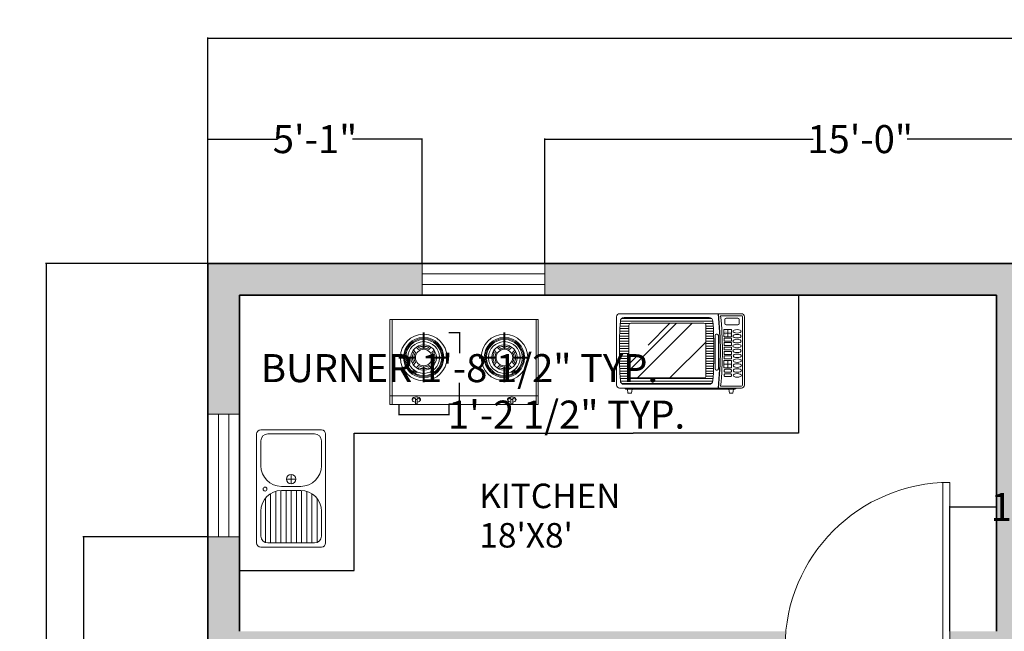
# Model space of a CAD drawing. Units: inches. Extents: x 638 to 1303, y 1 to 699.
# Tile 11 of 21: x 644 to 924, y 525 to 699. Entities that reach past the tile are written whole.
import ezdxf

# ---------------------------------------------------------------- set-up
doc = ezdxf.new("R2010")
doc.units = ezdxf.units.IN
doc.header["$MEASUREMENT"] = 0
for name, color, linetype, lineweight in [('A-ANNO-DIMS', 2, 'Continuous', 18), ('A-AREA-IDEN', 7, 'Continuous', 18), ('A-DOOR', 4, 'Continuous', 18), ('A-EQPM', 8, 'Continuous', 15), ('A-EQPM-PATT', 8, 'Continuous', 13), ('A-EQPM-TEXT', 8, 'Continuous', 13), ('A-FLOR-CASE', 8, 'Continuous', 25), ('A-FLOR-FIXT', 9, 'Continuous', 18), ('A-GLAZ', 4, 'Continuous', 18), ('A-WALL', 7, 'Continuous', 35)]:
    doc.layers.add(name, color=color, linetype=linetype, lineweight=lineweight)
doc.layers.add('A-WALL-PATT', color=143, linetype='Continuous', lineweight=13, true_color=0x7aafdf)
doc.styles.get("Standard").update_dxf_attribs({"font": 'arial.ttf'})
doc.dimstyles.get("Standard").update_dxf_attribs({"dimtxt": 8, "dimasz": 0.18, "dimexe": 0.18, "dimexo": 0.0625, "dimgap": 0.09, "dimtad": 0, "dimtih": 1, "dimtoh": 1, "dimdec": 4, "dimzin": 0, "dimdsep": 46, "dimlunit": 3, "dimtxsty": 'Standard', "dimcen": 0.09, "dimadec": 0, "dimazin": 0, "dimtfac": 1, "dimtdec": 4, "dimtofl": 0, "dimtmove": 0, "dimatfit": 3, "dimfxl": 1, "dimtolj": 1, "dimtzin": 0, "dimarcsym": 0})

# ---------------------------------------------------------------- blocks, each defined once
blk = doc.blocks.new('*D1')
at = {"layer": 'A-ANNO-DIMS', "color": 0, "lineweight": -2, "transparency": 16777216}
for p, q in [((697.18, 629.82), (650.92, 629.82)), ((651.1, 629.64), (651.1, 339.99)), ((651.1, 42), (651.1, 331.64)), ((697.18, 41.82), (650.92, 41.82))]:
    blk.add_line(p, q, dxfattribs=at)
at = {"layer": 'A-ANNO-DIMS', "color": 0, "transparency": 16777216}
for points in [[(651.07, 629.64), (651.13, 629.64), (651.1, 629.82)], [(651.07, 42), (651.13, 42), (651.1, 41.82)]]:
    blk.add_solid(points, dxfattribs=at)
at = {"layer": 'Defpoints', "color": 0, "transparency": 16777216}
for p in [(697.24, 629.82), (651.1, 41.82), (697.24, 41.82)]:
    blk.add_point(p, dxfattribs=at)
at = {"layer": 'A-ANNO-DIMS', "color": 0, "transparency": 16777216, "insert": (651.1, 335.82), "char_height": 8, "attachment_point": 5}
blk.add_mtext("\\A1;49'", dxfattribs=at)
blk = doc.blocks.new('*D2')
at = {"layer": 'A-ANNO-DIMS', "color": 0, "lineweight": -2, "transparency": 16777216}
for p, q in [((697.24, 629.88), (697.24, 694.35)), ((697.42, 694.17), (934.76, 694.17)), ((1228.06, 694.17), (990.71, 694.17)), ((1228.24, 629.88), (1228.24, 694.35))]:
    blk.add_line(p, q, dxfattribs=at)
at = {"layer": 'A-ANNO-DIMS', "color": 0, "transparency": 16777216}
for points in [[(697.42, 694.2), (697.42, 694.14), (697.24, 694.17)], [(1228.06, 694.2), (1228.06, 694.14), (1228.24, 694.17)]]:
    blk.add_solid(points, dxfattribs=at)
at = {"layer": 'Defpoints', "color": 0, "transparency": 16777216}
for p in [(1228.24, 694.17), (697.24, 629.82), (1228.24, 629.82)]:
    blk.add_point(p, dxfattribs=at)
at = {"layer": 'A-ANNO-DIMS', "color": 0, "transparency": 16777216, "insert": (962.74, 694.17), "char_height": 8, "attachment_point": 5}
blk.add_mtext('\\A1;44\'-3.0000"', dxfattribs=at)
blk = doc.blocks.new('DOOR-SWING-47')
for p, q in [((45, 0), (45, 46.96)), ((47, 0), (47, 47)), ((0, 0), (47, 0))]:
    blk.add_line(p, q)
blk.add_arc((47, 0), 47, 90, 180)
blk = doc.blocks.new('WIN-35')
for p, q in [((35, 9), (0, 9)), ((0, 9), (0, 0)), ((35, 0), (35, 9)), ((0, 6), (35, 6)), ((0, 3), (35, 3)), ((0, 0), (35, 0))]:
    blk.add_line(p, q)
blk = doc.blocks.new('COOKTOP-BURNER-CONTROL')
for p, q in [((6.96, 15.95), (6.96, 20.42)), ((7.27, 15.95), (7.27, 20.42)), ((4.21, 14.59), (3.9, 14.91)), ((4.81, 14.68), (4.16, 15.33)), ((5.67, 15.53), (5.01, 16.19)), ((5.75, 16.13), (5.44, 16.45)), ((8.48, 16.13), (8.79, 16.45)), ((8.56, 15.53), (9.22, 16.19)), ((9.42, 14.68), (10.07, 15.33)), ((10.01, 14.59), (10.33, 14.91)), ((4.4, 13.38), (0, 13.38)), ((4.4, 13.08), (0, 13.08)), ((3.9, 11.55), (4.21, 11.87)), ((4.16, 11.13), (4.81, 11.78)), ((10.07, 11.13), (9.42, 11.78)), ((9.83, 13.38), (14.27, 13.38)), ((9.83, 13.08), (14.27, 13.08)), ((10.33, 11.55), (10.01, 11.87)), ((5.01, 10.28), (5.67, 10.93)), ((5.44, 10.02), (5.75, 10.33)), ((6.96, 10.52), (6.96, 6.17)), ((7.27, 10.52), (7.27, 6.17)), ((8.79, 10.02), (8.48, 10.33)), ((9.22, 10.28), (8.56, 10.93)), ((3.8, 1.13), (3.8, 1.35)), ((4.74, 1.14), (4.74, 1.48)), ((4.74, 0.12), (4.74, 1.14)), ((4.86, 1.26), (5.16, 1.26)), ((5.16, 0), (4.86, 0)), ((5.28, 1.14), (5.28, 1.47)), ((5.28, 1.14), (5.28, 0.12)), ((6.19, 1.13), (6.19, 1.35))]:
    blk.add_line(p, q)
for centre, radius in [((7.11, 13.23), 2.36), ((4.18, 9.32), 0.216), ((4.73, 8.96), 0.216)]:
    blk.add_circle(centre, radius)
for centre, radius, start, end in [((7.11, 13.23), 6.65, 91.3023, 178.6977), ((7.11, 13.23), 6.65, 1.3023, 88.6977), ((7.11, 13.23), 5.74, 91.5918, 178.4082), ((7.11, 13.23), 5.44, 91.5918, 178.4082), ((7.11, 13.23), 5.14, 91.6854, 178.3146), ((7.11, 13.23), 4.53, 91.9102, 178.0898), ((7.11, 13.23), 5.74, 1.5918, 88.4082), ((7.11, 13.23), 5.44, 1.5918, 88.4082), ((7.11, 13.23), 5.14, 1.6854, 88.3146), ((7.11, 13.23), 4.53, 1.9102, 88.0898), ((7.11, 13.23), 3.63, 92.388, 177.612), ((7.11, 13.23), 3.2, 154.8539, 177.2964), ((7.11, 13.23), 2.72, 147.8396, 176.8153), ((7.11, 13.23), 2.72, 93.1847, 122.1604), ((7.11, 13.23), 3.2, 92.7036, 115.1461), ((7.11, 16), 0.161, 200.5507, 339.4493), ((7.11, 13.23), 3.63, 2.388, 87.612), ((7.11, 13.23), 3.2, 64.8539, 87.2964), ((7.11, 13.23), 2.72, 57.8396, 86.8153), ((7.11, 13.23), 2.72, 3.1847, 32.1604), ((7.11, 13.23), 3.2, 2.7036, 25.1461), ((7.11, 13.23), 6.65, 181.3023, 268.6977), ((7.11, 13.23), 5.74, 181.5918, 268.4082), ((7.11, 13.23), 5.44, 181.5918, 268.4082), ((7.11, 13.23), 5.14, 181.6854, 268.3146), ((7.11, 13.23), 4.53, 181.9102, 268.0898), ((7.11, 13.23), 3.63, 182.388, 267.612), ((7.11, 13.23), 3.2, 182.7036, 205.1461), ((4.38, 13.23), 0.152, 276.7354, 83.2646), ((7.11, 13.23), 2.72, 183.1847, 212.1604), ((7.11, 13.23), 6.65, 271.3023, 358.6977), ((7.11, 13.23), 5.44, 271.5918, 358.4082), ((7.11, 13.23), 3.63, 272.388, 357.612), ((7.11, 13.23), 4.53, 271.9102, 358.0898), ((7.11, 13.23), 5.14, 271.6854, 358.3146), ((7.11, 13.23), 5.74, 271.5918, 358.4082), ((7.11, 13.23), 2.72, 327.8396, 356.8153), ((9.89, 13.23), 0.163, 111.7885, 248.2115), ((7.11, 13.23), 3.2, 334.8539, 357.2964), ((7.11, 13.23), 2.72, 237.8396, 266.8153), ((7.11, 13.23), 3.2, 244.8539, 267.2964), ((7.11, 10.46), 0.16, 18.751, 161.249), ((7.11, 13.23), 2.72, 273.1847, 302.1604), ((7.11, 13.23), 3.2, 272.7036, 295.1461), ((3.92, 1.12), 0.121, 131.3486, 194.6729), ((5, -0.11), 1.75, 103.3075, 131.3486), ((4.62, 1.48), 0.121, 0, 103.3075), ((4.86, 1.14), 0.121, 90, 180), ((4.86, 0.12), 0.121, 180, 270), ((5.16, 1.14), 0.121, 0, 90), ((5.16, 0.12), 0.121, 270, 360), ((5.4, 1.47), 0.121, 75.624, 180), ((5, -0.11), 1.75, 50.3889, 75.624), ((6.03, 1.1), 0.16, 327.8142, 59.9251)]:
    blk.add_arc(centre, radius, start, end)
for start_param, end_param in [(3.311147, 6.113631), (0.167831, 1.359229), (1.807364, 2.885846)]:
    blk.add_ellipse((5, 1.22), major_axis=(-1.21, 0), ratio=0.647058, start_param=start_param, end_param=end_param)
blk = doc.blocks.new('*D38')
at = {"layer": 'A-ANNO-DIMS', "color": 0, "lineweight": -2, "transparency": 16777216}
for p, q in [((766.03, 610.16), (769.21, 610.16)), ((769.03, 609.98), (769.03, 604.18)), ((769.03, 589.93), (769.03, 595.73)), ((766.03, 589.75), (769.21, 589.75))]:
    blk.add_line(p, q, dxfattribs=at)
at = {"layer": 'A-ANNO-DIMS', "color": 0, "transparency": 16777216}
for points in [[(769, 609.98), (769.06, 609.98), (769.03, 610.16)], [(769, 589.93), (769.06, 589.93), (769.03, 589.75)]]:
    blk.add_solid(points, dxfattribs=at)
at = {"layer": 'Defpoints', "color": 0, "transparency": 16777216}
for p in [(765.97, 610.16), (769.03, 610.16), (765.97, 589.75)]:
    blk.add_point(p, dxfattribs=at)
at = {"layer": 'A-ANNO-DIMS', "color": 0, "transparency": 16777216, "insert": (769.03, 599.95), "char_height": 8, "attachment_point": 5}
blk.add_mtext('\\A1;BURNER 1\'-8 1/2" TYP.', dxfattribs=at)
blk = doc.blocks.new('*D39')
at = {"layer": 'A-ANNO-DIMS', "color": 0, "lineweight": -2, "transparency": 16777216}
for p, q in [((751.7, 589.68), (751.7, 586.5)), ((765.97, 589.68), (765.97, 586.5)), ((751.88, 586.68), (765.79, 586.68)), ((765.97, 586.68), (766.15, 586.68))]:
    blk.add_line(p, q, dxfattribs=at)
at = {"layer": 'A-ANNO-DIMS', "color": 0, "transparency": 16777216}
for points in [[(751.88, 586.71), (751.88, 586.65), (751.7, 586.68)], [(765.79, 586.71), (765.79, 586.65), (765.97, 586.68)]]:
    blk.add_solid(points, dxfattribs=at)
at = {"layer": 'Defpoints', "color": 0, "transparency": 16777216}
for p in [(751.7, 589.75), (765.97, 589.75), (765.97, 586.68)]:
    blk.add_point(p, dxfattribs=at)
at = {"layer": 'A-ANNO-DIMS', "color": 0, "transparency": 16777216, "insert": (799.57, 586.68), "char_height": 8, "attachment_point": 5}
blk.add_mtext('\\A1;1\'-2 1/2" TYP.', dxfattribs=at)
blk = doc.blocks.new('*D51')
at = {"layer": 'A-ANNO-DIMS', "color": 0, "lineweight": -2, "transparency": 16777216}
for p, q in [((697.24, 629.88), (697.24, 665.5)), ((697.42, 665.32), (717.07, 665.32)), ((758.18, 665.32), (738.52, 665.32)), ((758.36, 629.88), (758.36, 665.5))]:
    blk.add_line(p, q, dxfattribs=at)
at = {"layer": 'A-ANNO-DIMS', "color": 0, "transparency": 16777216}
for points in [[(697.42, 665.35), (697.42, 665.29), (697.24, 665.32)], [(758.18, 665.35), (758.18, 665.29), (758.36, 665.32)]]:
    blk.add_solid(points, dxfattribs=at)
at = {"layer": 'Defpoints', "color": 0, "transparency": 16777216}
for p in [(758.36, 665.32), (697.24, 629.82), (758.36, 629.82)]:
    blk.add_point(p, dxfattribs=at)
at = {"layer": 'A-ANNO-DIMS', "color": 0, "transparency": 16777216, "insert": (727.8, 665.32), "char_height": 8, "attachment_point": 5}
blk.add_mtext('\\A1;5\'-1"', dxfattribs=at)
blk = doc.blocks.new('*D52')
at = {"layer": 'A-ANNO-DIMS', "color": 0, "lineweight": -2, "transparency": 16777216}
for p, q in [((793.36, 629.88), (793.36, 665.5)), ((793.54, 665.32), (869.9, 665.32)), ((973.17, 665.32), (896.8, 665.32)), ((973.35, 629.88), (973.35, 665.5))]:
    blk.add_line(p, q, dxfattribs=at)
at = {"layer": 'A-ANNO-DIMS', "color": 0, "transparency": 16777216}
for points in [[(793.54, 665.35), (793.54, 665.29), (793.36, 665.32)], [(973.17, 665.35), (973.17, 665.29), (973.35, 665.32)]]:
    blk.add_solid(points, dxfattribs=at)
at = {"layer": 'Defpoints', "color": 0, "transparency": 16777216}
for p in [(973.35, 665.32), (793.36, 629.82), (973.35, 629.82)]:
    blk.add_point(p, dxfattribs=at)
at = {"layer": 'A-ANNO-DIMS', "color": 0, "transparency": 16777216, "insert": (883.35, 665.32), "char_height": 8, "attachment_point": 5}
blk.add_mtext('\\A1;15\'-0"', dxfattribs=at)
blk = doc.blocks.new('*D59')
at = {"layer": 'A-ANNO-DIMS', "color": 0, "lineweight": -2, "transparency": 16777216}
for p, q in [((697.18, 551.77), (661.56, 551.77)), ((661.74, 551.59), (661.74, 520.91)), ((661.74, 481.88), (661.74, 512.57)), ((697.18, 481.7), (661.56, 481.7))]:
    blk.add_line(p, q, dxfattribs=at)
at = {"layer": 'A-ANNO-DIMS', "color": 0, "transparency": 16777216}
for points in [[(661.71, 551.59), (661.77, 551.59), (661.74, 551.77)], [(661.71, 481.88), (661.77, 481.88), (661.74, 481.7)]]:
    blk.add_solid(points, dxfattribs=at)
at = {"layer": 'Defpoints', "color": 0, "transparency": 16777216}
for p in [(661.74, 551.77), (697.24, 551.77), (697.24, 481.7)]:
    blk.add_point(p, dxfattribs=at)
at = {"layer": 'A-ANNO-DIMS', "color": 0, "transparency": 16777216, "insert": (661.74, 516.74), "char_height": 8, "attachment_point": 5}
blk.add_mtext('\\A1;5\'-10"', dxfattribs=at)
blk = doc.blocks.new('*D68')
at = {"layer": 'A-ANNO-DIMS', "color": 0, "lineweight": -2, "transparency": 16777216}
for p, q in [((908.94, 524.88), (908.94, 560.5)), ((909.12, 560.32), (922.06, 560.32)), ((922.24, 524.88), (922.24, 560.5)), ((922.24, 560.32), (922.42, 560.32))]:
    blk.add_line(p, q, dxfattribs=at)
at = {"layer": 'A-ANNO-DIMS', "color": 0, "transparency": 16777216}
for points in [[(909.12, 560.35), (909.12, 560.29), (908.94, 560.32)], [(922.06, 560.35), (922.06, 560.29), (922.24, 560.32)]]:
    blk.add_solid(points, dxfattribs=at)
at = {"layer": 'Defpoints', "color": 0, "transparency": 16777216}
for p in [(922.24, 560.32), (908.94, 524.82), (922.24, 524.82)]:
    blk.add_point(p, dxfattribs=at)
at = {"layer": 'A-ANNO-DIMS', "color": 0, "transparency": 16777216, "insert": (942.09, 560.32), "char_height": 8, "attachment_point": 5}
blk.add_mtext('\\A1;1\'-1 1/2"', dxfattribs=at)

msp = doc.modelspace()

# ---------------------------------------------------------------- hatches: boundary and pattern name
at = {"layer": 'A-EQPM-PATT'}
h = msp.add_hatch(dxfattribs=at)
h.set_pattern_fill('ANSI31', color=256, scale=5.71925, angle=-45, style=0)
h.paths.add_polyline_path([(815.99748, 595.32966), (840.27522, 595.32966), (840.33134, 595.33113), (840.38731, 595.33554), (840.44297, 595.34286), (840.49817, 595.3531), (840.55276, 595.3662), (840.60659, 595.38215), (840.65952, 595.40089), (840.71139, 595.42237), (840.76206, 595.44654), (840.8114, 595.47333), (840.85927, 595.50267), (840.90553, 595.53446), (840.95007, 595.56864), (840.99277, 595.6051), (841.03349, 595.64375), (841.07214, 595.68447), (841.1086, 595.72716), (841.14277, 595.7717), (841.17457, 595.81797), (841.20391, 595.86584), (841.2307, 595.91518), (841.25487, 595.96585), (841.27635, 596.01772), (841.29509, 596.07064), (841.31104, 596.12447), (841.32414, 596.17906), (841.33437, 596.23427), (841.3417, 596.28993), (841.34611, 596.3459), (841.34758, 596.40202), (841.58905, 602.04806), (841.58905, 607.69925), (841.34758, 613.34529), (841.34611, 613.40141), (841.3417, 613.45738), (841.33437, 613.51304), (841.32414, 613.56825), (841.31104, 613.62284), (841.29509, 613.67667), (841.27635, 613.72959), (841.25487, 613.78146), (841.2307, 613.83213), (841.20391, 613.88147), (841.17457, 613.92934), (841.14277, 613.97561), (841.1086, 614.02015), (841.07214, 614.06284), (841.03349, 614.10356), (840.99277, 614.14221), (840.95007, 614.17867), (840.90553, 614.21285), (840.85927, 614.24465), (840.8114, 614.27398), (840.76206, 614.30077), (840.71139, 614.32494), (840.65952, 614.34642), (840.60659, 614.36516), (840.55276, 614.38111), (840.49817, 614.39421), (840.44297, 614.40445), (840.38731, 614.41177), (840.33134, 614.41618), (840.27522, 614.41765), (815.99748, 614.41765), (815.94136, 614.41618), (815.88539, 614.41177), (815.82973, 614.40445), (815.77453, 614.39421), (815.71994, 614.38111), (815.66611, 614.36516), (815.61318, 614.34642), (815.56132, 614.32494), (815.51064, 614.30077), (815.4613, 614.27398), (815.41343, 614.24465), (815.36717, 614.21285), (815.32263, 614.17867), (815.27993, 614.14221), (815.23921, 614.10356), (815.20057, 614.06284), (815.1641, 614.02015), (815.12993, 613.97561), (815.09813, 613.92934), (815.06879, 613.88147), (815.042, 613.83213), (815.01783, 613.78146), (814.99635, 613.72959), (814.97761, 613.67667), (814.96166, 613.62284), (814.94856, 613.56825), (814.93833, 613.51304), (814.931, 613.45738), (814.92659, 613.40141), (814.92512, 613.34529), (814.68365, 607.69925), (814.68365, 602.04806), (814.92512, 596.40202), (814.92659, 596.3459), (814.931, 596.28993), (814.93833, 596.23427), (814.94856, 596.17906), (814.96166, 596.12447), (814.97761, 596.07064), (814.99635, 596.01772), (815.01783, 595.96585), (815.042, 595.91518), (815.06879, 595.86584), (815.09813, 595.81797), (815.12993, 595.7717), (815.1641, 595.72716), (815.20057, 595.68447), (815.23921, 595.64375), (815.27993, 595.6051), (815.32263, 595.56864), (815.36717, 595.53446), (815.41343, 595.50267), (815.4613, 595.47333), (815.51064, 595.44654), (815.56132, 595.42237), (815.61318, 595.40089), (815.66611, 595.38215), (815.71994, 595.3662), (815.77453, 595.3531), (815.82973, 595.34286), (815.88539, 595.33554), (815.94136, 595.33113)])
h.paths.add_polyline_path([(817.95732, 612.75288), (838.77542, 612.75288), (838.80439, 612.75214), (838.83328, 612.74994), (838.86203, 612.74628), (838.89055, 612.74117), (838.91878, 612.73462), (838.94664, 612.72665), (838.97406, 612.71728), (839.00097, 612.70653), (839.0273, 612.69443), (839.05298, 612.68101), (839.07795, 612.66631), (839.10215, 612.65037), (839.1255, 612.63322), (839.14796, 612.6149), (839.16946, 612.59548), (839.18995, 612.57499), (839.20938, 612.55349), (839.22769, 612.53103), (839.24484, 612.50767), (839.26078, 612.48348), (839.27548, 612.45851), (839.2889, 612.43282), (839.301, 612.40649), (839.31175, 612.37958), (839.32112, 612.35217), (839.32909, 612.32431), (839.33564, 612.29608), (839.34075, 612.26756), (839.34441, 612.23881), (839.34661, 612.20992), (839.34735, 612.18095), (839.34735, 597.71228), (839.34661, 597.68331), (839.34441, 597.65442), (839.34075, 597.62567), (839.33564, 597.59715), (839.32909, 597.56892), (839.32112, 597.54106), (839.31175, 597.51364), (839.301, 597.48673), (839.2889, 597.4604), (839.27548, 597.43472), (839.26078, 597.40975), (839.24484, 597.38555), (839.22769, 597.3622), (839.20938, 597.33974), (839.18995, 597.31824), (839.16946, 597.29775), (839.14796, 597.27832), (839.1255, 597.26001), (839.10215, 597.24286), (839.07795, 597.22692), (839.05298, 597.21222), (839.0273, 597.1988), (839.00097, 597.1867), (838.97406, 597.17595), (838.94664, 597.16658), (838.91878, 597.15861), (838.89055, 597.15206), (838.86203, 597.14695), (838.83328, 597.14329), (838.80439, 597.14109), (838.77542, 597.14035), (817.95732, 597.14035), (817.92739, 597.14114), (817.89754, 597.14349), (817.86785, 597.14739), (817.83841, 597.15285), (817.8093, 597.15984), (817.78059, 597.16834), (817.75236, 597.17834), (817.7247, 597.1898), (817.69768, 597.20269), (817.67136, 597.21698), (817.64583, 597.23262), (817.62115, 597.24958), (817.5974, 597.26781), (817.57463, 597.28725), (817.55291, 597.30786), (817.5323, 597.32958), (817.51285, 597.35235), (817.49463, 597.37611), (817.47767, 597.40078), (817.46202, 597.42631), (817.44773, 597.45263), (817.43484, 597.47965), (817.42339, 597.50732), (817.41339, 597.53554), (817.40489, 597.56425), (817.3979, 597.59337), (817.39244, 597.62281), (817.38853, 597.65249), (817.38618, 597.68234), (817.3854, 597.71228), (817.3854, 612.18095), (817.38618, 612.21088), (817.38853, 612.24073), (817.39244, 612.27042), (817.3979, 612.29986), (817.40489, 612.32898), (817.41339, 612.35769), (817.42339, 612.38591), (817.43484, 612.41358), (817.44773, 612.4406), (817.46202, 612.46691), (817.47767, 612.49244), (817.49463, 612.51712), (817.51285, 612.54088), (817.5323, 612.56364), (817.55291, 612.58536), (817.57463, 612.60598), (817.5974, 612.62542), (817.62115, 612.64365), (817.64583, 612.66061), (817.67136, 612.67625), (817.69768, 612.69054), (817.7247, 612.70343), (817.75236, 612.71489), (817.78059, 612.72489), (817.8093, 612.73339), (817.83841, 612.74038), (817.86785, 612.74584), (817.89754, 612.74974), (817.92739, 612.75209)], flags=0)
at = {"layer": 'A-WALL-PATT'}
h = msp.add_hatch(color=256, dxfattribs=at)
h.dxf.hatch_style = 1
h.paths.add_polyline_path([(973.34524, 629.81895), (793.35541, 629.81895), (793.35541, 620.81895), (850.23798, 620.81895), (922.23798, 620.81895), (922.23798, 524.81895), (908.94335, 524.81895), (908.94335, 520.31895), (926.73798, 520.31895), (926.73798, 544.31895), (979.3571, 544.31895), (979.3571, 548.81895), (926.73798, 548.81895), (926.73798, 620.81895), (973.34524, 620.81895)])
h.paths.add_polyline_path([(758.35541, 629.81895), (697.23798, 629.81895), (697.23798, 586.77451), (706.23798, 586.77451), (706.23798, 620.81895), (758.35541, 620.81895)])
h.paths.add_polyline_path([(1075.85281, 629.81895), (1003.34524, 629.81895), (1003.34524, 620.81895), (1046.73798, 620.81895), (1046.73798, 560.81895), (1046.73798, 548.81895), (1026.3571, 548.81895), (1026.3571, 544.31895), (1046.73798, 544.31895), (1046.73798, 486.87457), (1051.23798, 486.87457), (1051.23798, 556.31895), (1162.89753, 556.31895), (1162.89753, 560.81895), (1051.23798, 560.81895), (1051.23798, 620.81895), (1075.85281, 620.81895)])
h.paths.add_polyline_path([(1228.23798, 629.81895), (1105.85281, 629.81895), (1105.85281, 620.81895), (1219.23798, 620.81895), (1219.23798, 560.81895), (1197.89753, 560.81895), (1197.89753, 556.31895), (1219.23798, 556.31895), (1219.23798, 498.80084), (1228.23798, 498.80084)])
h.paths.add_polyline_path([(1051.23798, 439.87457), (1046.73798, 439.87457), (1046.73798, 407.81895), (1219.23798, 407.81895), (1219.23798, 381.66175), (1228.23798, 381.66175), (1228.23798, 451.80084), (1219.23798, 451.80084), (1219.23798, 412.31895), (1051.23798, 412.31895)])
h.paths.add_polyline_path([(1228.23798, 346.66175), (1219.23798, 346.66175), (1219.23798, 335.81895), (1046.73798, 335.81895), (1046.73798, 273.56895), (1051.23798, 273.56895), (1051.23798, 331.31895), (1219.23798, 331.31895), (1219.23798, 308.99654), (1228.23798, 308.99654)])
h.paths.add_polyline_path([(1228.23798, 261.99654), (1219.23798, 261.99654), (1219.23798, 211.31895), (1051.23798, 211.31895), (1051.23798, 226.56895), (1046.73798, 226.56895), (1046.73798, 211.31895), (983.84714, 211.31895), (983.84714, 206.81895), (1219.23798, 206.81895), (1219.23798, 166.83987), (1228.23798, 166.83987)])
h.paths.add_polyline_path([(1228.23798, 119.83987), (1219.23798, 119.83987), (1219.23798, 50.81895), (1197.89277, 50.81895), (1197.89277, 41.81895), (1228.23798, 41.81895)])
h.paths.add_polyline_path([(1162.89277, 50.81895), (1069.02949, 50.81895), (1069.02949, 41.81895), (1162.89277, 41.81895)])
h.paths.add_polyline_path([(1010.02949, 50.81895), (941.89631, 50.81895), (917.77455, 50.81895), (917.77455, 41.81895), (941.89631, 41.81895), (1010.02949, 41.81895)])
h.paths.add_polyline_path([(882.77455, 50.81895), (854.73798, 50.81895), (854.73798, 145.50379), (850.23798, 145.50379), (850.23798, 50.81895), (793.49755, 50.81895), (793.49755, 41.81895), (882.77455, 41.81895)])
h.paths.add_polyline_path([(746.49755, 50.81895), (706.23798, 50.81895), (706.23798, 96.57416), (697.23798, 96.57416), (697.23798, 41.81895), (746.49755, 41.81895)])
h.paths.add_polyline_path([(706.23798, 206.81895), (714.01165, 206.81895), (714.01165, 211.31895), (706.23798, 211.31895), (706.23798, 251.21966), (697.23798, 251.21966), (697.23798, 143.57416), (706.23798, 143.57416)])
h.paths.add_polyline_path([(923.84714, 211.31895), (854.73798, 211.31895), (854.73798, 397.8313), (850.23798, 397.8313), (850.23798, 388.31895), (747.9539, 388.31895), (747.9539, 383.81895), (850.23798, 383.81895), (850.23798, 311.81895), (706.23798, 311.81895), (706.23798, 342.78787), (697.23798, 342.78787), (697.23798, 281.21966), (706.23798, 281.21966), (706.23798, 307.31895), (850.23798, 307.31895), (850.23798, 211.31895), (749.01165, 211.31895), (749.01165, 206.81895), (850.23798, 206.81895), (850.23798, 192.50379), (854.73798, 192.50379), (854.73798, 206.81895), (923.84714, 206.81895)])
h.paths.add_polyline_path([(706.23798, 434.70471), (697.23798, 434.70471), (697.23798, 372.78787), (706.23798, 372.78787), (706.23798, 383.81895), (712.9539, 383.81895), (712.9539, 388.31895), (706.23798, 388.31895)])
h.paths.add_polyline_path([(706.23798, 520.31895), (850.23798, 520.31895), (850.23798, 444.8313), (854.73798, 444.8313), (854.73798, 520.31895), (861.94335, 520.31895), (861.94335, 524.81895), (706.23798, 524.81895), (706.23798, 551.77451), (697.23798, 551.77451), (697.23798, 481.70471), (706.23798, 481.70471)])

# ---------------------------------------------------------------- linework, layer by layer
at = {"layer": 'A-EQPM'}
for p, q in [((849.45508, 615.49001), (814.71065, 615.49001)), ((749.17396, 613.78425), (749.17396, 589.61118)), ((791.47682, 613.78425), (749.17396, 613.78425)), ((749.77828, 613.78425), (749.77828, 589.61118)), ((790.8725, 589.61118), (790.8725, 613.78425)), ((791.47682, 589.61118), (791.47682, 613.78425)), ((813.85277, 614.63212), (813.85277, 595.11519)), ((840.27522, 614.41765), (815.99748, 614.41765)), ((817.3854, 599.20787), (830.93041, 612.75288)), ((817.95732, 612.75288), (838.77542, 612.75288)), ((819.83759, 597.14035), (835.45012, 612.75288)), ((822.85874, 606.53018), (829.08144, 612.75288)), ((849.45508, 614.91808), (843.53981, 614.91808)), ((844.73806, 613.84156), (844.73806, 612.65573)), ((848.48867, 614.19902), (845.09551, 614.19902)), ((848.84612, 612.65573), (848.84612, 613.84156)), ((849.74104, 595.11519), (849.74104, 614.63212)), ((850.31296, 595.11519), (850.31296, 614.63212)), ((817.3854, 597.71228), (817.3854, 612.18095)), ((839.34735, 612.18095), (839.34735, 597.71228)), ((844.48841, 609.04465), (844.48841, 610.85858)), ((844.48841, 609.95161), (846.67941, 609.95161)), ((844.6314, 611.00156), (846.53643, 611.00156)), ((845.09551, 612.29828), (848.48867, 612.29828)), ((845.58391, 611.00156), (845.58391, 608.90167)), ((846.67941, 610.85858), (846.67941, 609.04465)), ((829.08245, 597.14035), (839.34735, 607.40526)), ((841.95141, 599.71814), (841.95141, 609.30894)), ((842.30886, 609.66639), (842.53673, 609.66639)), ((842.89418, 609.30894), (842.89418, 599.71814)), ((844.50537, 607.78978), (844.50537, 608.34392)), ((844.50537, 606.53492), (844.50537, 607.08905)), ((846.53643, 608.90167), (844.6314, 608.90167)), ((844.64835, 608.4869), (846.53067, 608.4869)), ((846.53067, 607.6468), (844.64835, 607.6468)), ((844.64835, 607.23203), (846.53067, 607.23203)), ((846.67365, 608.34392), (846.67365, 607.78978)), ((846.67365, 607.08905), (846.67365, 606.53492)), ((844.50537, 605.28006), (844.50537, 605.83419)), ((844.50537, 604.02519), (844.50537, 604.57932)), ((846.53067, 606.39194), (844.64835, 606.39194)), ((844.64835, 605.97717), (846.53067, 605.97717)), ((846.53067, 605.13708), (844.64835, 605.13708)), ((844.64835, 604.72231), (846.53067, 604.72231)), ((846.67365, 605.83419), (846.67365, 605.28006)), ((846.67365, 604.57932), (846.67365, 604.02519)), ((817.3854, 601.05684), (819.46896, 603.1404)), ((844.48841, 600.17483), (844.48841, 601.98876)), ((844.50537, 602.77033), (844.50537, 603.32446)), ((844.6314, 602.13174), (846.53643, 602.13174)), ((846.53067, 603.88221), (844.64835, 603.88221)), ((844.64835, 603.46744), (846.53067, 603.46744)), ((846.53067, 602.62735), (844.64835, 602.62735)), ((845.58391, 602.13174), (845.58391, 600.03185)), ((846.67365, 603.32446), (846.67365, 602.77033)), ((846.67941, 601.98876), (846.67941, 600.17483)), ((842.53673, 599.36068), (842.30886, 599.36068)), ((844.48841, 601.0818), (846.67941, 601.0818)), ((846.53643, 600.03185), (844.6314, 600.03185)), ((844.93139, 599.61708), (846.25958, 599.61708)), ((846.25958, 598.77699), (844.93139, 598.77699)), ((838.77542, 597.14035), (817.95732, 597.14035)), ((844.93139, 598.36222), (846.25958, 598.36222)), ((846.25958, 597.52212), (844.93139, 597.52212)), ((814.71065, 594.2573), (849.45508, 594.2573)), ((815.99748, 595.32966), (840.27522, 595.32966)), ((816.17621, 594.2573), (847.98952, 594.2573)), ((816.53366, 593.97134), (816.17621, 594.2573)), ((816.53366, 593.97134), (818.67838, 593.97134)), ((816.93401, 593.97134), (817.10559, 592.82749)), ((818.27803, 593.97134), (818.10646, 592.82749)), ((818.67838, 593.97134), (845.48735, 593.97134)), ((843.53981, 594.82923), (849.45508, 594.82923)), ((845.48735, 593.97134), (847.63207, 593.97134)), ((845.8877, 593.97134), (846.05927, 592.82749)), ((847.23172, 593.97134), (847.06014, 592.82749)), ((847.98952, 594.2573), (847.63207, 593.97134)), ((749.17396, 592.02849), (791.47682, 592.02849)), ((817.10559, 592.82749), (818.10646, 592.82749)), ((846.05927, 592.82749), (847.06014, 592.82749)), ((749.17396, 589.61118), (791.47682, 589.61118))]:
    msp.add_line(p, q, dxfattribs=at)
for centre, radius, start, end in [((814.71065, 614.63212), 0.85789, 90, 180), ((744.65775, 604.87366), 98.73319, 353.832679, 6.167321), ((744.65775, 604.87366), 98.81898, 353.832679, 6.167321), ((849.45508, 614.63212), 0.85789, 360, 90), ((946.87562, 604.87366), 132.22217, 176.3264736, 183.6735264), ((815.99748, 613.34529), 1.07236, 90, 180), ((817.95732, 612.18095), 0.57192, 90, 180), ((838.77542, 612.18095), 0.57192, 360, 90), ((840.27522, 613.34529), 1.07236, 0, 90), ((709.39279, 604.87366), 132.22645, 356.3265928, 3.6734072), ((744.65775, 604.87366), 99.3909, 354.1997969, 5.8002031), ((845.09551, 613.84156), 0.35745, 90, 180), ((845.09551, 612.65573), 0.35745, 180, 270), ((848.48867, 613.84156), 0.35745, 0, 90), ((848.48867, 612.65573), 0.35745, 270, 0), ((849.45508, 614.63212), 0.28596, 0, 90), ((844.6314, 610.85858), 0.14298, 90, 180), ((846.53643, 610.85858), 0.14298, 360, 90), ((842.30886, 609.30894), 0.35745, 90, 180), ((842.53673, 609.30894), 0.35745, 0, 90), ((844.6314, 609.04465), 0.14298, 180, 270), ((844.64835, 608.34392), 0.14298, 90, 180), ((844.64835, 607.78978), 0.14298, 180, 270), ((844.64835, 607.08905), 0.14298, 90, 180), ((846.53067, 608.34392), 0.14298, 360, 90), ((846.53067, 607.78978), 0.14298, 270, 360), ((846.53067, 607.08905), 0.14298, 360, 90), ((846.53643, 609.04465), 0.14298, 270, 0), ((844.64835, 606.53492), 0.14298, 180, 270), ((844.64835, 605.83419), 0.14298, 90, 180), ((844.64835, 605.28006), 0.14298, 180, 270), ((844.64835, 604.57932), 0.14298, 90, 180), ((846.53067, 606.53492), 0.14298, 270, 0), ((846.53067, 605.83419), 0.14298, 360, 90), ((846.53067, 605.28006), 0.14298, 270, 0), ((846.53067, 604.57932), 0.14298, 360, 90), ((844.6314, 601.98876), 0.14298, 90, 180), ((844.64835, 604.02519), 0.14298, 180, 270), ((844.64835, 603.32446), 0.14298, 90, 180), ((844.64835, 602.77033), 0.14298, 180, 270), ((846.53067, 604.02519), 0.14298, 270, 0), ((846.53067, 603.32446), 0.14298, 360, 90), ((846.53067, 602.77033), 0.14298, 270, 0), ((846.53643, 601.98876), 0.14298, 0, 90), ((842.30886, 599.71814), 0.35745, 180, 270), ((842.53673, 599.71814), 0.35745, 270, 0), ((844.6314, 600.17483), 0.14298, 180, 270), ((844.93139, 599.19703), 0.42005, 89.9996313, 270.0003687), ((846.25958, 599.19703), 0.42005, 269.9996313, 90.0003687), ((846.53643, 600.17483), 0.14298, 270, 0), ((815.99748, 596.40202), 1.07236, 180, 270), ((817.95732, 597.71228), 0.57192, 180, 270), ((838.77542, 597.71228), 0.57192, 270, 0), ((840.27522, 596.40202), 1.07236, 270, 0), ((844.93139, 597.94217), 0.42005, 89.9996313, 270.0003687), ((846.25958, 597.94217), 0.42005, 269.9996313, 90.0003687), ((814.71065, 595.11519), 0.85789, 180, 270), ((849.45508, 595.11519), 0.28596, 270, 0), ((849.45508, 595.11519), 0.85789, 270, 0)]:
    msp.add_arc(centre, radius, start, end, dxfattribs=at)
for centre in [(848.23155, 610.46339), (848.23155, 609.06523), (848.23155, 609.06523), (848.23155, 607.66708), (848.24609, 606.26889), (848.24609, 606.26889), (848.24609, 604.87073), (848.26062, 603.47261), (848.26062, 603.47261), (848.26062, 602.07446), (848.27516, 600.67626), (848.27516, 600.67626), (848.27516, 599.27811), (848.27516, 597.87995)]:
    msp.add_ellipse(centre, major_axis=(-1.18691, 0), ratio=0.42447819, dxfattribs=at)
at = {"layer": 'A-FLOR-CASE'}
for p, q in [((865.77593, 620.81895), (865.77593, 581.38577)), ((738.98109, 542.21474), (738.98109, 581.38577)), ((738.98109, 581.38577), (818.56383, 581.38577)), ((865.77593, 581.38577), (818.56383, 581.38577)), ((706.23798, 542.21474), (706.23798, 542.21474)), ((706.23798, 542.21474), (738.98109, 542.21474))]:
    msp.add_line(p, q, dxfattribs=at)
at = {"layer": 'A-FLOR-FIXT'}
for p, q in [((712.32784, 582.33234), (729.65064, 582.33234)), ((711.14674, 550.04894), (711.14674, 581.15124)), ((712.32784, 572.09614), (712.32784, 579.18274)), ((714.29634, 581.15124), (727.68214, 581.15124)), ((729.65064, 572.09614), (729.65064, 579.18274)), ((730.83174, 550.04894), (730.83174, 581.15124)), ((719.64794, 568.26109), (722.33054, 568.26109)), ((720.98924, 569.60239), (720.98924, 566.91979)), ((716.57797, 550.04894), (716.57797, 564.77834)), ((718.05435, 550.04894), (718.05435, 565.00806)), ((718.23334, 566.19064), (723.74514, 566.19064)), ((718.23334, 565.00954), (723.74514, 565.00954)), ((719.53072, 550.04894), (719.53072, 565.00954)), ((721.0071, 550.04894), (721.0071, 565.00954)), ((722.48347, 550.04894), (722.48347, 565.00954)), ((723.95985, 550.04894), (723.95985, 565.00421)), ((725.43622, 550.04894), (725.43622, 564.75646)), ((713.62522, 550.15974), (713.62522, 562.81891)), ((715.1016, 550.04894), (715.1016, 564.12188)), ((726.9126, 550.04894), (726.9126, 564.07679)), ((728.38897, 550.18821), (728.38897, 562.72997)), ((712.32784, 559.10404), (712.32784, 552.01744)), ((729.65064, 559.10404), (729.65064, 552.01744)), ((712.32784, 548.86784), (729.65064, 548.86784)), ((714.29634, 550.04894), (727.68214, 550.04894))]:
    msp.add_line(p, q, dxfattribs=at)
for centre, radius in [((720.98924, 568.26109), 1.3413), ((713.53938, 565.42486), 0.5539)]:
    msp.add_circle(centre, radius, dxfattribs=at)
for centre, radius, start, end in [((712.32784, 581.15124), 1.1811, 90, 180), ((729.65064, 581.15124), 1.1811, 0, 90), ((714.29634, 579.18274), 1.9685, 90, 180), ((727.68214, 579.18274), 1.9685, 0, 90), ((718.23334, 572.09614), 5.9055, 180, 270), ((723.74514, 572.09614), 5.9055, 270, 0), ((718.23334, 559.10404), 5.9055, 90, 180), ((723.74514, 559.10404), 5.9055, 0, 90), ((714.29634, 552.01744), 1.9685, 180, 270), ((727.68214, 552.01744), 1.9685, 270, 0), ((712.32784, 550.04894), 1.1811, 180, 270), ((729.65064, 550.04894), 1.1811, 270, 0)]:
    msp.add_arc(centre, radius, start, end, dxfattribs=at)
at = {"layer": 'A-WALL'}
for p, q in [((697.23798, 41.81895), (697.23798, 629.81895)), ((1228.23798, 629.81895), (697.23798, 629.81895)), ((850.23798, 620.81895), (706.23798, 620.81895)), ((706.23798, 524.81895), (706.23798, 620.81895)), ((922.23798, 620.81895), (850.23798, 620.81895)), ((922.23798, 524.81895), (922.23798, 620.81895))]:
    msp.add_line(p, q, dxfattribs=at)

# ---------------------------------------------------------------- block references
at = {"layer": 'A-DOOR'}
msp.add_blockref('DOOR-SWING-47', (861.943, 520.319), dxfattribs=at)
at = {"layer": 'A-EQPM'}
msp.add_blockref('COOKTOP-BURNER-CONTROL', (751.697, 589.745), dxfattribs=at)
at = {"layer": 'A-EQPM', "extrusion": (0, 0, -1), "zscale": -1}
msp.add_blockref('COOKTOP-BURNER-CONTROL', (-788.95378, 589.745), dxfattribs=at)
at = {"layer": 'A-GLAZ'}
msp.add_blockref('WIN-35', (758.35564, 620.819), dxfattribs=at)
at = {"layer": 'A-GLAZ', "rotation": 269.9999999999997}
msp.add_blockref('WIN-35', (697.23803, 586.77428), dxfattribs=at)

# ---------------------------------------------------------------- texts
at = {"layer": 'A-AREA-IDEN'}
for s, p in [('KITCHEN', (774.69014, 559.97453)), ("18'X8'", (774.69014, 548.72964))]:
    msp.add_text(s, height=7, dxfattribs=at).set_placement(p)
at = {"layer": 'A-EQPM-TEXT'}
for s, height, p in [('10', 0.285962, (844.70146, 610.36349)), ('分', 0.28596, (845.19168, 610.36349)), ('1', 0.28596, (845.79597, 610.36349)), ('分', 0.28596, (846.01385, 610.36349)), ('10', 0.285962, (844.70146, 609.32752)), ('秒', 0.28596, (845.19168, 609.32752)), ('1', 0.28596, (845.79597, 609.32752)), ('秒', 0.28596, (846.01385, 609.32752))]:
    msp.add_text(s, height=height, dxfattribs=at).set_placement(p)

# ---------------------------------------------------------------- dimensions: what is measured, and where the dimension line sits
at = {"layer": 'A-ANNO-DIMS'}
for base, p1, p2, override, picture, middle in [((1228.23798, 694.16557), (697.23798, 629.81895), (1228.23798, 629.81895), {"dimclrd": 0, "dimclre": 0, "dimclrt": 0}, '*D2', (962.73798, 694.16557)), ((758.35541, 665.31895), (697.23798, 629.81895), (758.35541, 629.81895), {"dimdec": 1, "dimlfac": 1, "dimrnd": 0, "dimzin": 1, "dimdsep": 46, "dimlunit": 4, "dimfrac": 2}, '*D51', (727.79669, 665.31895)), ((973.34524, 665.31895), (793.35541, 629.81895), (973.34524, 629.81895), {"dimdec": 1, "dimlfac": 1, "dimrnd": 0, "dimzin": 1, "dimdsep": 46, "dimlunit": 4, "dimfrac": 2}, '*D52', (883.35032, 665.31895))]:
    dim = msp.add_linear_dim(base=base, p1=p1, p2=p2, dimstyle='Standard', override=override, dxfattribs=at)
    dim.commit()
    dim.dimension.update_dxf_attribs({"geometry": picture, "text_midpoint": middle})
for base, p1, p2, angle, override, picture, middle in [((651.10111, 41.81895), (697.23798, 629.81895), (697.23798, 41.81895), 90, {"dimclrd": 0, "dimclre": 0, "dimclrt": 0}, '*D1', (651.10111, 335.81895)), ((922.23798, 560.31895), (908.94335, 524.81895), (922.23798, 524.81895), 0, {"dimdec": 1, "dimlfac": 1, "dimrnd": 0, "dimzin": 1, "dimdsep": 46, "dimlunit": 4, "dimfrac": 2}, '*D68', (942.08506, 560.31895)), ((661.73798, 551.77451), (697.23798, 481.70471), (697.23798, 551.77451), 90, {"dimdec": 1, "dimlfac": 1, "dimrnd": 0, "dimzin": 1, "dimdsep": 46, "dimlunit": 4, "dimfrac": 2}, '*D59', (661.73798, 516.73961))]:
    dim = msp.add_linear_dim(base=base, p1=p1, p2=p2, angle=angle, dimstyle='Standard', override=override, dxfattribs=at)
    dim.commit()
    dim.dimension.update_dxf_attribs({"geometry": picture, "text_midpoint": middle})
dim = msp.add_linear_dim(base=(769.03413, 610.16204), p1=(765.9716, 589.74515), p2=(765.9716, 610.16204), angle=90, text='BURNER <> TYP.', dimstyle='Standard', override={"dimdec": 1, "dimlfac": 1, "dimrnd": 0, "dimzin": 1, "dimdsep": 46, "dimlunit": 4, "dimfrac": 2}, dxfattribs=at)
dim.commit()
dim.dimension.update_dxf_attribs({"geometry": '*D38', "text_midpoint": (769.03413, 599.9536)})
dim = msp.add_linear_dim(base=(765.9716, 586.68262), p1=(751.69711, 589.74515), p2=(765.9716, 589.74515), text='<> TYP.', dimstyle='Standard', override={"dimdec": 1, "dimlfac": 1, "dimrnd": 0, "dimzin": 1, "dimdsep": 46, "dimlunit": 4, "dimfrac": 2}, dxfattribs=at)
dim.commit()
dim.dimension.update_dxf_attribs({"geometry": '*D39', "text_midpoint": (799.56765, 586.68262)})

doc.saveas('drawing.dxf')
